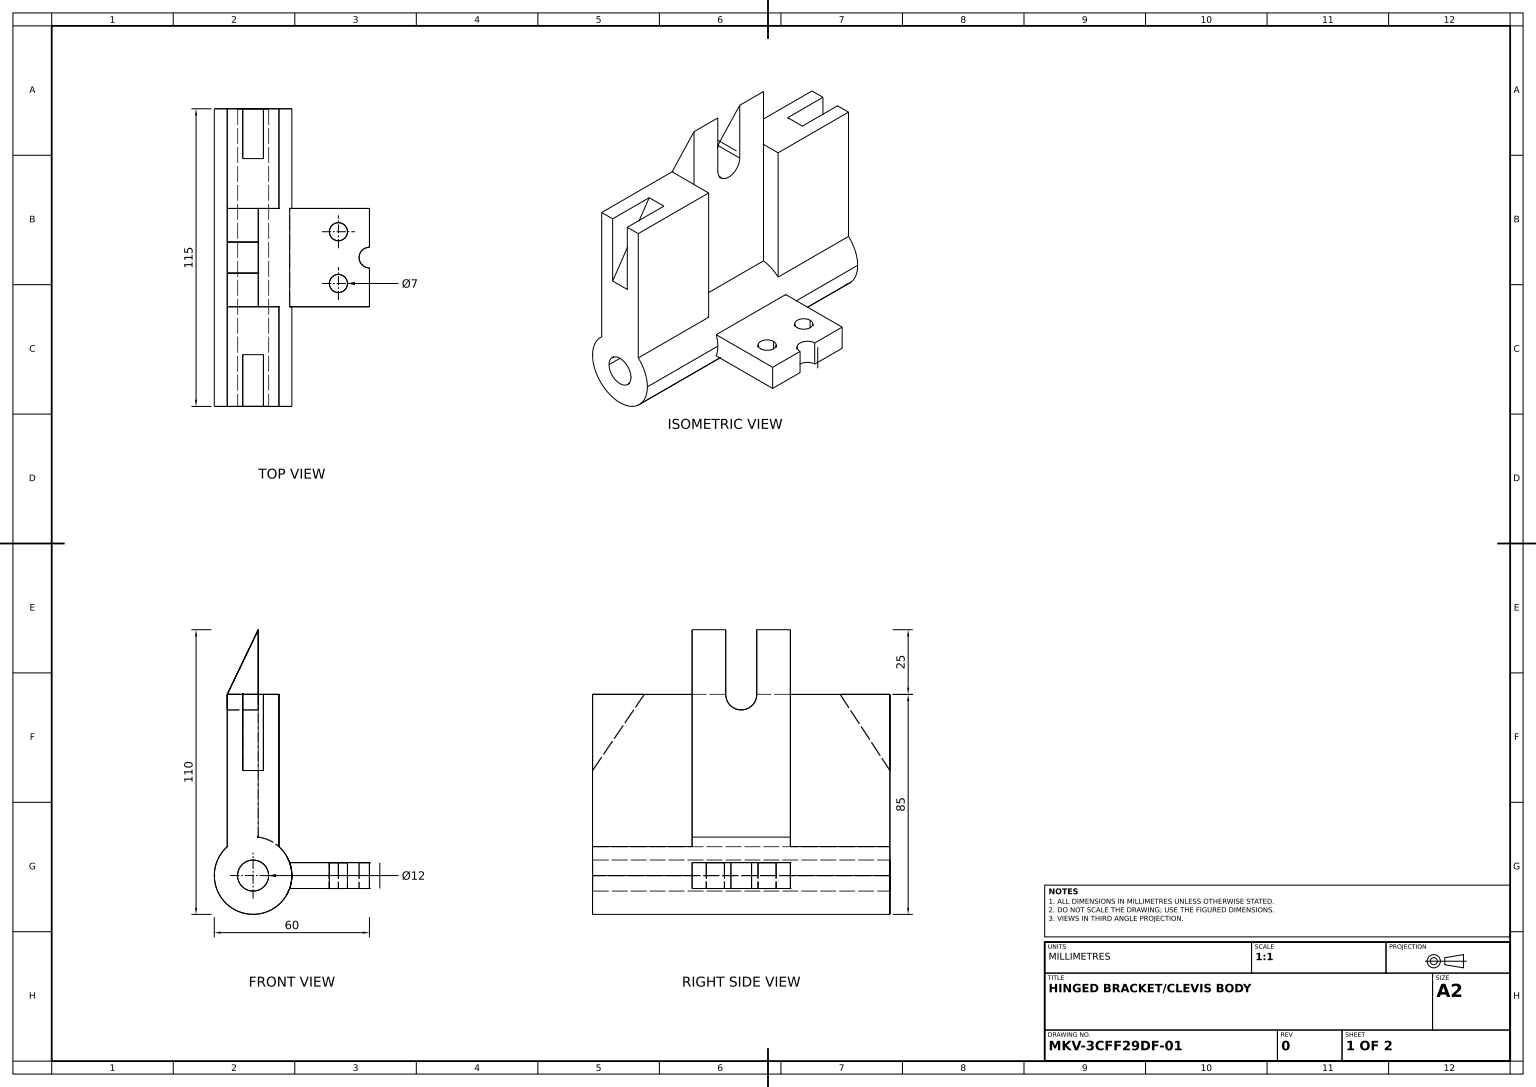
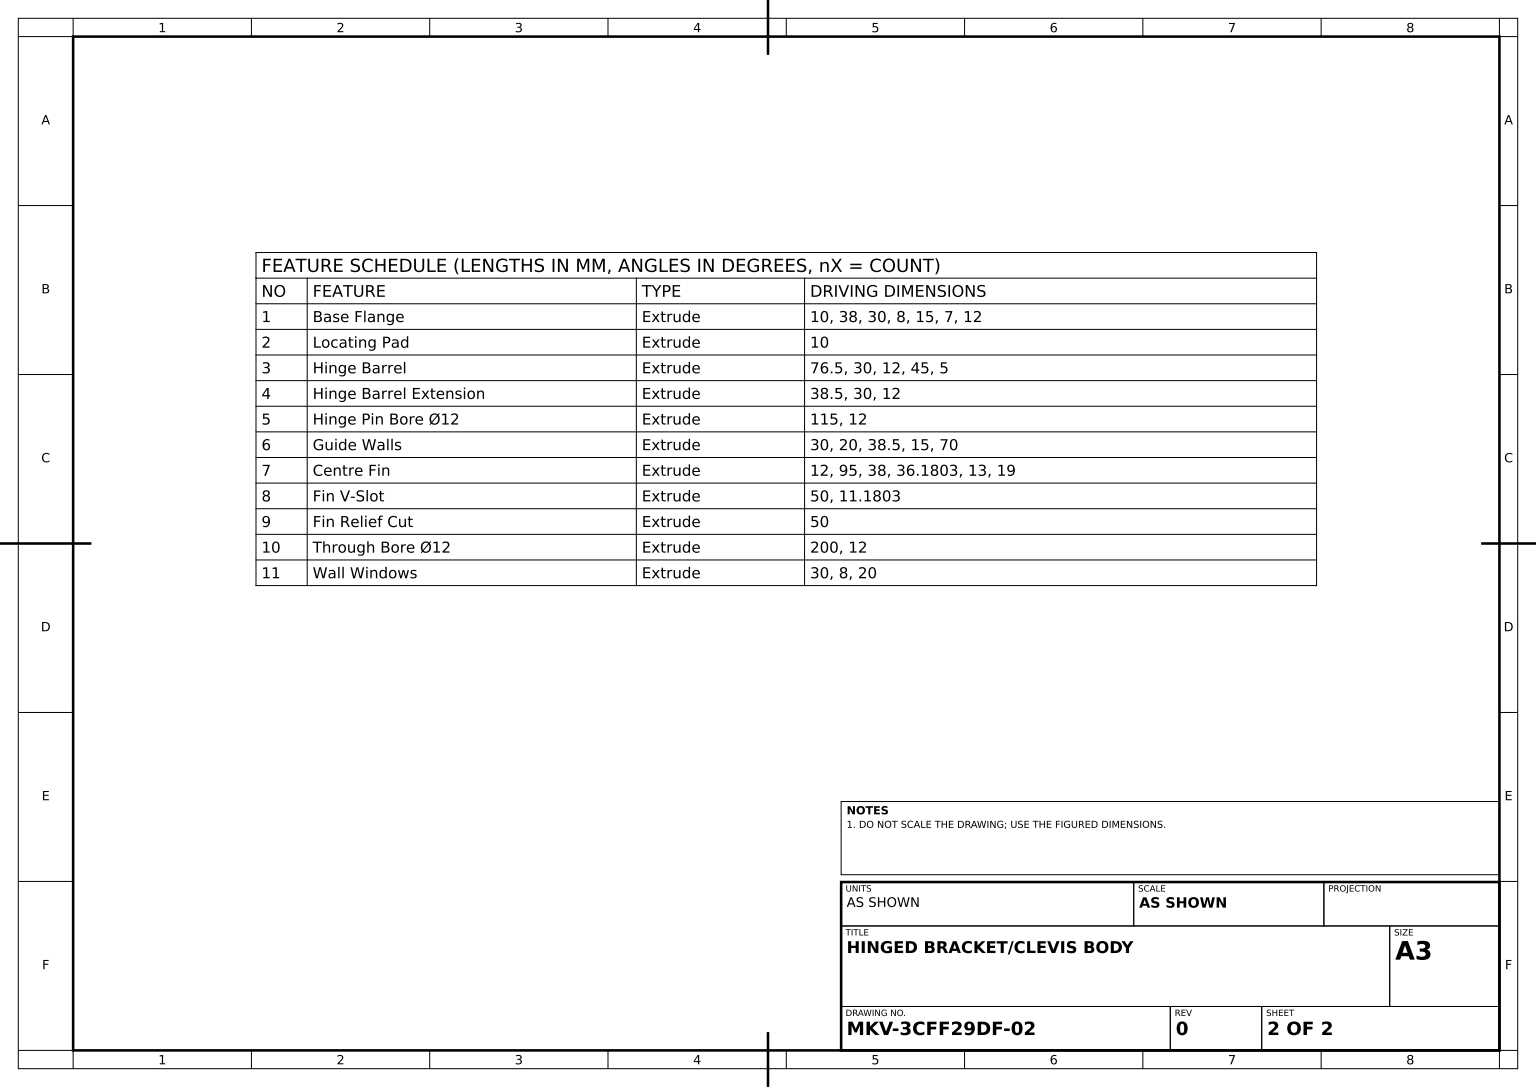
from build123d import *

# Parameters (mm, degrees)
BASE_FLANGE_SKETCH_R         = 3.5
BASE_FLANGE_DEPTH            = 10
LOCATING_PAD_SKETCH_W        = 38
LOCATING_PAD_SKETCH_H        = 10
LOCATING_PAD_DEPTH           = 10
HINGE_BARREL_SKETCH_R        = 15
HINGE_BARREL_SKETCH_R_2      = 6
HINGE_BARREL_DEPTH           = 76.5
HINGE_START                  = 38.5
BARREL_EXTENSION_SKETCH_R    = 15
BARREL_EXTENSION_SKETCH_R_2  = 6
HINGE_BARREL_EXTENSION_DEPTH = 38.5
PIN_BORE_SKETCH_R            = 6
HINGE_PIN_BORE_12_DEPTH      = 115
GUIDE_WALLS_SKETCH_W         = 38.5
GUIDE_WALLS_SKETCH_H         = 70
GUIDE_WALLS_DEPTH            = 10
CENTRE_FIN_DEPTH             = 12
FIN_V_SLOT_SKETCH_W          = 12
FIN_V_SLOT_SKETCH_H          = 11.180339887
FIN_V_SLOT_DEPTH             = 50
FIN_RELIEF_CUT_DEPTH         = 50
THROUGH_BORE_SKETCH_R        = 6
THROUGH_BORE_12_DEPTH        = 200
WALL_WINDOWS_DEPTH           = 4


with BuildPart() as part:
    # Base Flange Sketch → Base Flange (new body)
    with BuildSketch(Plane(origin=(0, 0, 0), x_dir=(1, 0, 0), z_dir=(0, 1, 0))):
        with BuildLine():
            Line((15, -4), (15, -19))
            Line((15, -19), (-15, -19))
            Line((-15, -19), (-15, 19))
            Line((-15, 19), (15, 19))
            Line((15, 19), (15, 4))
            ThreePointArc((15, 4), (11, 0), (15, -4))
        make_face()
        with Locations(Location((3, 10, 0), (0, 0, 270))):
            Circle(BASE_FLANGE_SKETCH_R, mode=Mode.SUBTRACT)
        with Locations(Location((3, -10, 0), (0, 0, 270))):
            Circle(BASE_FLANGE_SKETCH_R, mode=Mode.SUBTRACT)
    extrude(amount=BASE_FLANGE_DEPTH)

    # Locating Pad Sketch → Locating Pad (add)
    with BuildSketch(Plane.ZY.offset(15)):
        with Locations((0, 5)):
            Rectangle(LOCATING_PAD_SKETCH_W, LOCATING_PAD_SKETCH_H)
    extrude(amount=LOCATING_PAD_DEPTH)

    # Hinge Barrel Sketch → Hinge Barrel (add)
    with BuildSketch(Plane.XY.offset(19)):
        with Locations((-30, 5)):
            Circle(HINGE_BARREL_SKETCH_R)
        with Locations((-30, 5)):
            Circle(HINGE_BARREL_SKETCH_R_2, mode=Mode.SUBTRACT)
    extrude(amount=-HINGE_BARREL_DEPTH)

    # Barrel Extension Sketch → Hinge Barrel Extension (add)
    with BuildSketch(Plane.XY.offset(19).offset(HINGE_START)):
        with Locations((-30, 5)):
            Circle(BARREL_EXTENSION_SKETCH_R)
        with Locations((-30, 5)):
            Circle(BARREL_EXTENSION_SKETCH_R_2, mode=Mode.SUBTRACT)
    extrude(amount=-HINGE_BARREL_EXTENSION_DEPTH)

    # Pin Bore Sketch → Hinge Pin Bore Ø12 (cut)
    with BuildSketch(Plane.XY.offset(57.5)):
        with Locations((-30, 5)):
            Circle(PIN_BORE_SKETCH_R)
    extrude(amount=-HINGE_PIN_BORE_12_DEPTH, mode=Mode.SUBTRACT)

    # Guide Walls Sketch → Guide Walls (add, symmetric)
    with BuildSketch(Plane(origin=(-30, 0, 0), x_dir=(0, 0, -1), z_dir=(1, 0, 0))):
        with Locations((38.25, 40)):
            Rectangle(GUIDE_WALLS_SKETCH_W, GUIDE_WALLS_SKETCH_H)
        with Locations((-38.25, 40)):
            Rectangle(GUIDE_WALLS_SKETCH_W, GUIDE_WALLS_SKETCH_H)
    extrude(amount=GUIDE_WALLS_DEPTH, both=True)

    # Centre Fin Sketch → Centre Fin (add)
    with BuildSketch(Plane.ZY.offset(40)):
        with BuildLine():
            Line((-19, 16.180339887), (19, 16.180339887))
            Line((19, 16.180339887), (19, 111.180339887))
            Line((19, 111.180339887), (6, 111.180339887))
            Line((6, 111.180339887), (6, 75))
            ThreePointArc((6, 75), (0, 69), (-6, 75))
            Line((-6, 75), (-6, 111.180339887))
            Line((-6, 111.180339887), (-19, 111.180339887))
            Line((-19, 111.180339887), (-19, 16.180339887))
        make_face()
    extrude(amount=-CENTRE_FIN_DEPTH)

    # Fin V-Slot Sketch → Fin V-Slot (cut)
    with BuildSketch(Plane.XY.offset(19)):
        with Locations((-34, 105.590169944)):
            Rectangle(FIN_V_SLOT_SKETCH_W, FIN_V_SLOT_SKETCH_H)
    extrude(amount=-FIN_V_SLOT_DEPTH, mode=Mode.SUBTRACT)

    # Fin Relief Sketch → Fin Relief Cut (cut)
    with BuildSketch(Plane.XY.offset(19)):
        Polygon((-40, 75), (-28, 100), (-40, 100), align=None)
    extrude(amount=-FIN_RELIEF_CUT_DEPTH, mode=Mode.SUBTRACT)

    # Through Bore Sketch → Through Bore Ø12 (cut)
    with BuildSketch(Plane.XY.offset(57.5)):
        with Locations((-30, 5)):
            Circle(THROUGH_BORE_SKETCH_R)
    extrude(amount=-THROUGH_BORE_12_DEPTH, mode=Mode.SUBTRACT)

    # Wall Window Sketch → Wall Windows (cut, symmetric)
    with BuildSketch(Plane(origin=(-30, 0, 0), x_dir=(0, 0, -1), z_dir=(1, 0, 0))):
        Polygon((57.5, 75), (38.25, 75), (57.5, 45.590169944), align=None)
        Polygon((-57.5, 75), (-57.5, 45.590169944), (-37.5, 75), align=None)
    extrude(amount=WALL_WINDOWS_DEPTH, both=True, mode=Mode.SUBTRACT)


solid = part.part
